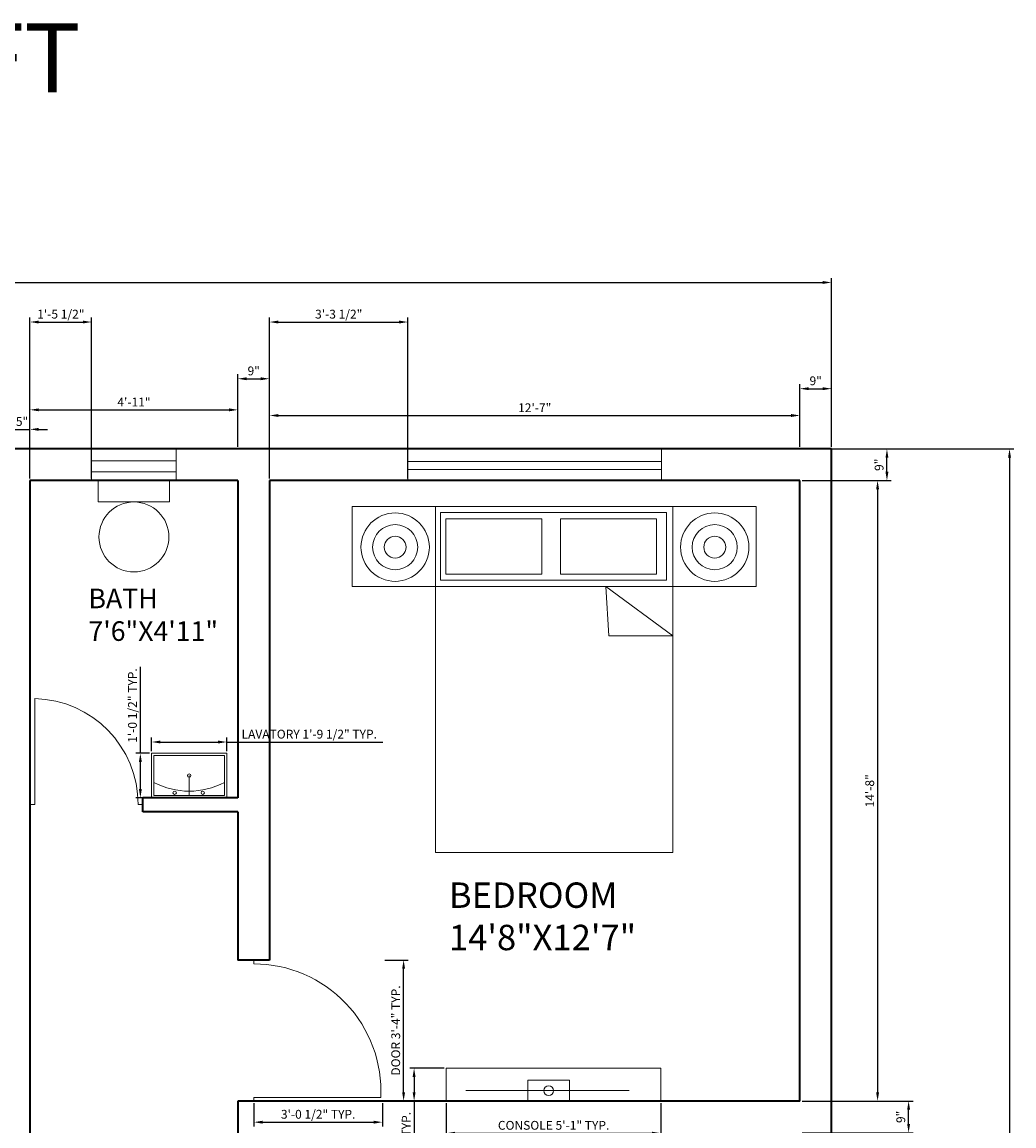
# Model space of a CAD drawing. Units: inches. Extents: x 808 to 1433, y 803 to 1556.
# Tile 4 of 4: x 1151 to 1433, y 1243 to 1556. Entities that reach past the tile are written whole.
import ezdxf

# ---------------------------------------------------------------- set-up
doc = ezdxf.new("R2010")
doc.units = ezdxf.units.IN
for name, color, linetype, lineweight in [('A-ANNO-DIMS', 7, 'Continuous', 13), ('A-AREA-IDEN', 7, 'Continuous', 18), ('A-WALL', 7, 'Continuous', 35)]:
    doc.layers.add(name, color=color, linetype=linetype, lineweight=lineweight)
for name, color, linetype, lineweight, true_color in [('A-ANNO-TITL', 244, 'Continuous', 25, 0x991b1e), ('A-DOOR', 251, 'Continuous', 18, 0x636466), ('A-FLOR-FIXT', 251, 'Continuous', 18, 0x636466), ('A-FURN', 251, 'Continuous', 13, 0x636466), ('A-GLAZ', 251, 'Continuous', 18, 0x636466)]:
    doc.layers.add(name, color=color, linetype=linetype, lineweight=lineweight, true_color=true_color)
doc.styles.get("Standard").update_dxf_attribs({"font": 'arial.ttf'})
doc.dimstyles.new('ISO-25', dxfattribs={"dimtxt": 2.5, "dimasz": 2.5, "dimexe": 1.25, "dimexo": 0.625, "dimtad": 1, "dimdec": 0, "dimlunit": 3, "dimtxsty": 'Standard', "dimcen": 2.5, "dimadec": 0, "dimazin": 0, "dimtfac": 1, "dimtdec": 0, "dimtmove": 0, "dimatfit": 3, "dimfxl": 1, "dimarcsym": 0})

# ---------------------------------------------------------------- blocks, each defined once
blk = doc.blocks.new('*D1')
at = {"layer": 'A-ANNO-DIMS', "color": 0, "lineweight": -2, "transparency": 16777216}
for p, q in [((854.88, 1435.69), (854.88, 1483.54)), ((857.38, 1482.29), (1378.38, 1482.29)), ((1380.88, 1435.69), (1380.88, 1483.54))]:
    blk.add_line(p, q, dxfattribs=at)
at = {"layer": 'A-ANNO-DIMS', "color": 0, "transparency": 16777216}
for points in [[(857.38, 1482.7), (857.38, 1481.87), (854.88, 1482.29)], [(1378.38, 1482.7), (1378.38, 1481.87), (1380.88, 1482.29)]]:
    blk.add_solid(points, dxfattribs=at)
at = {"layer": 'Defpoints', "color": 0, "transparency": 16777216}
for p in [(1380.88, 1482.29), (854.88, 1435.07), (1380.88, 1435.07)]:
    blk.add_point(p, dxfattribs=at)
at = {"layer": 'A-ANNO-DIMS', "color": 0, "transparency": 16777216, "insert": (1117.88, 1484.19), "char_height": 2.5, "attachment_point": 5}
blk.add_mtext('43\'-10"', dxfattribs=at)
blk = doc.blocks.new('*D2')
at = {"layer": 'A-ANNO-DIMS', "color": 0, "lineweight": -2, "transparency": 16777216}
for p, q in [((1381.5, 1435.07), (1432.64, 1435.07)), ((1431.39, 1432.57), (1431.39, 843.57)), ((1381.5, 841.07), (1432.64, 841.07))]:
    blk.add_line(p, q, dxfattribs=at)
at = {"layer": 'A-ANNO-DIMS', "color": 0, "transparency": 16777216}
for points in [[(1430.97, 1432.57), (1431.8, 1432.57), (1431.39, 1435.07)], [(1430.97, 843.57), (1431.8, 843.57), (1431.39, 841.07)]]:
    blk.add_solid(points, dxfattribs=at)
at = {"layer": 'Defpoints', "color": 0, "transparency": 16777216}
for p in [(1380.88, 1435.07), (1380.88, 841.07), (1431.39, 841.07)]:
    blk.add_point(p, dxfattribs=at)
at = {"layer": 'A-ANNO-DIMS', "color": 0, "transparency": 16777216, "insert": (1429.48, 1138.07), "char_height": 2.5, "attachment_point": 5, "rotation": 90}
blk.add_mtext('49\'-6"', dxfattribs=at)
blk = doc.blocks.new('*D7')
at = {"layer": 'A-ANNO-DIMS', "color": 0, "lineweight": -2, "transparency": 16777216}
for p, q in [((1146.38, 1440.62), (1143.88, 1440.62)), ((1148.88, 1435.69), (1148.88, 1441.87)), ((1148.88, 1440.62), (1153.38, 1440.62)), ((1153.38, 1435.69), (1153.38, 1441.87)), ((1155.88, 1440.62), (1158.38, 1440.62))]:
    blk.add_line(p, q, dxfattribs=at)
at = {"layer": 'A-ANNO-DIMS', "color": 0, "transparency": 16777216}
for points in [[(1146.38, 1441.04), (1146.38, 1440.2), (1148.88, 1440.62)], [(1155.88, 1441.04), (1155.88, 1440.2), (1153.38, 1440.62)]]:
    blk.add_solid(points, dxfattribs=at)
at = {"layer": 'Defpoints', "color": 0, "transparency": 16777216}
for p in [(1153.38, 1440.62), (1148.88, 1435.07), (1153.38, 1435.07)]:
    blk.add_point(p, dxfattribs=at)
at = {"layer": 'A-ANNO-DIMS', "color": 0, "transparency": 16777216, "insert": (1151.13, 1442.52), "char_height": 2.5, "attachment_point": 5}
blk.add_mtext('5"', dxfattribs=at)
blk = doc.blocks.new('*D8')
at = {"layer": 'A-ANNO-DIMS', "color": 0, "lineweight": -2, "transparency": 16777216}
for p, q in [((1153.38, 1435.69), (1153.38, 1447.4)), ((1212.38, 1435.69), (1212.38, 1447.4)), ((1155.88, 1446.15), (1209.88, 1446.15))]:
    blk.add_line(p, q, dxfattribs=at)
at = {"layer": 'A-ANNO-DIMS', "color": 0, "transparency": 16777216}
for points in [[(1155.88, 1446.57), (1155.88, 1445.74), (1153.38, 1446.15)], [(1209.88, 1446.57), (1209.88, 1445.74), (1212.38, 1446.15)]]:
    blk.add_solid(points, dxfattribs=at)
at = {"layer": 'Defpoints', "color": 0, "transparency": 16777216}
for p in [(1212.38, 1446.15), (1153.38, 1435.07), (1212.38, 1435.07)]:
    blk.add_point(p, dxfattribs=at)
at = {"layer": 'A-ANNO-DIMS', "color": 0, "transparency": 16777216, "insert": (1182.88, 1448.03), "char_height": 2.5, "attachment_point": 5}
blk.add_mtext('4\'-11"', dxfattribs=at)
blk = doc.blocks.new('*D9')
at = {"layer": 'A-ANNO-DIMS', "color": 0, "lineweight": -2, "transparency": 16777216}
for p, q in [((1212.38, 1435.69), (1212.38, 1456.23)), ((1221.38, 1435.69), (1221.38, 1456.23)), ((1214.88, 1454.98), (1218.88, 1454.98))]:
    blk.add_line(p, q, dxfattribs=at)
at = {"layer": 'A-ANNO-DIMS', "color": 0, "transparency": 16777216}
for points in [[(1214.88, 1455.39), (1214.88, 1454.56), (1212.38, 1454.98)], [(1218.88, 1455.39), (1218.88, 1454.56), (1221.38, 1454.98)]]:
    blk.add_solid(points, dxfattribs=at)
at = {"layer": 'Defpoints', "color": 0, "transparency": 16777216}
for p in [(1221.38, 1454.98), (1212.38, 1435.07), (1221.38, 1435.07)]:
    blk.add_point(p, dxfattribs=at)
at = {"layer": 'A-ANNO-DIMS', "color": 0, "transparency": 16777216, "insert": (1216.88, 1456.88), "char_height": 2.5, "attachment_point": 5}
blk.add_mtext('9"', dxfattribs=at)
blk = doc.blocks.new('*D10')
at = {"layer": 'A-ANNO-DIMS', "color": 0, "lineweight": -2, "transparency": 16777216}
for p, q in [((1371.88, 1435.69), (1371.88, 1453.41)), ((1380.88, 1435.69), (1380.88, 1453.41)), ((1374.38, 1452.16), (1378.38, 1452.16))]:
    blk.add_line(p, q, dxfattribs=at)
at = {"layer": 'A-ANNO-DIMS', "color": 0, "transparency": 16777216}
for points in [[(1374.38, 1452.57), (1374.38, 1451.74), (1371.88, 1452.16)], [(1378.38, 1452.57), (1378.38, 1451.74), (1380.88, 1452.16)]]:
    blk.add_solid(points, dxfattribs=at)
at = {"layer": 'Defpoints', "color": 0, "transparency": 16777216}
for p in [(1380.88, 1452.16), (1371.88, 1435.07), (1380.88, 1435.07)]:
    blk.add_point(p, dxfattribs=at)
at = {"layer": 'A-ANNO-DIMS', "color": 0, "transparency": 16777216, "insert": (1376.38, 1454.06), "char_height": 2.5, "attachment_point": 5}
blk.add_mtext('9"', dxfattribs=at)
blk = doc.blocks.new('*D11')
at = {"layer": 'A-ANNO-DIMS', "color": 0, "lineweight": -2, "transparency": 16777216}
for p, q in [((1221.38, 1435.69), (1221.38, 1445.8)), ((1223.88, 1444.55), (1369.38, 1444.55)), ((1371.88, 1435.69), (1371.88, 1445.8))]:
    blk.add_line(p, q, dxfattribs=at)
at = {"layer": 'A-ANNO-DIMS', "color": 0, "transparency": 16777216}
for points in [[(1223.88, 1444.97), (1223.88, 1444.13), (1221.38, 1444.55)], [(1369.38, 1444.97), (1369.38, 1444.13), (1371.88, 1444.55)]]:
    blk.add_solid(points, dxfattribs=at)
at = {"layer": 'Defpoints', "color": 0, "transparency": 16777216}
for p in [(1371.88, 1444.55), (1221.38, 1435.07), (1371.88, 1435.07)]:
    blk.add_point(p, dxfattribs=at)
at = {"layer": 'A-ANNO-DIMS', "color": 0, "transparency": 16777216, "insert": (1296.63, 1446.43), "char_height": 2.5, "attachment_point": 5}
blk.add_mtext('12\'-7"', dxfattribs=at)
blk = doc.blocks.new('*D20')
at = {"layer": 'A-ANNO-DIMS', "color": 0, "lineweight": -2, "transparency": 16777216}
for p, q in [((1372.5, 1435.07), (1397.84, 1435.07)), ((1396.59, 1428.57), (1396.59, 1432.57)), ((1372.5, 1426.07), (1397.84, 1426.07))]:
    blk.add_line(p, q, dxfattribs=at)
at = {"layer": 'A-ANNO-DIMS', "color": 0, "transparency": 16777216}
for points in [[(1396.18, 1432.57), (1397.01, 1432.57), (1396.59, 1435.07)], [(1396.18, 1428.57), (1397.01, 1428.57), (1396.59, 1426.07)]]:
    blk.add_solid(points, dxfattribs=at)
at = {"layer": 'Defpoints', "color": 0, "transparency": 16777216}
for p in [(1371.88, 1435.07), (1396.59, 1435.07), (1371.88, 1426.07)]:
    blk.add_point(p, dxfattribs=at)
at = {"layer": 'A-ANNO-DIMS', "color": 0, "transparency": 16777216, "insert": (1394.69, 1430.57), "char_height": 2.5, "attachment_point": 5, "rotation": 90}
blk.add_mtext('9"', dxfattribs=at)
blk = doc.blocks.new('*D21')
at = {"layer": 'A-ANNO-DIMS', "color": 0, "lineweight": -2, "transparency": 16777216}
for p, q in [((1372.5, 1250.07), (1404, 1250.07)), ((1402.75, 1243.57), (1402.75, 1247.57)), ((1372.5, 1241.07), (1404, 1241.07))]:
    blk.add_line(p, q, dxfattribs=at)
at = {"layer": 'A-ANNO-DIMS', "color": 0, "transparency": 16777216}
for points in [[(1402.33, 1247.57), (1403.16, 1247.57), (1402.75, 1250.07)], [(1402.33, 1243.57), (1403.16, 1243.57), (1402.75, 1241.07)]]:
    blk.add_solid(points, dxfattribs=at)
at = {"layer": 'Defpoints', "color": 0, "transparency": 16777216}
for p in [(1371.88, 1250.07), (1402.75, 1250.07), (1371.88, 1241.07)]:
    blk.add_point(p, dxfattribs=at)
at = {"layer": 'A-ANNO-DIMS', "color": 0, "transparency": 16777216, "insert": (1400.85, 1245.57), "char_height": 2.5, "attachment_point": 5, "rotation": 90}
blk.add_mtext('9"', dxfattribs=at)
blk = doc.blocks.new('*D26')
at = {"layer": 'A-ANNO-DIMS', "color": 0, "lineweight": -2, "transparency": 16777216}
for p, q in [((1381.5, 1426.07), (1395.19, 1426.07)), ((1393.94, 1423.57), (1393.94, 1252.57)), ((1381.5, 1250.07), (1395.19, 1250.07))]:
    blk.add_line(p, q, dxfattribs=at)
at = {"layer": 'A-ANNO-DIMS', "color": 0, "transparency": 16777216}
for points in [[(1393.52, 1423.57), (1394.36, 1423.57), (1393.94, 1426.07)], [(1393.52, 1252.57), (1394.36, 1252.57), (1393.94, 1250.07)]]:
    blk.add_solid(points, dxfattribs=at)
at = {"layer": 'Defpoints', "color": 0, "transparency": 16777216}
for p in [(1380.88, 1426.07), (1380.88, 1250.07), (1393.94, 1250.07)]:
    blk.add_point(p, dxfattribs=at)
at = {"layer": 'A-ANNO-DIMS', "color": 0, "transparency": 16777216, "insert": (1392.04, 1338.07), "char_height": 2.5, "attachment_point": 5, "rotation": 90}
blk.add_mtext('14\'-8"', dxfattribs=at)
blk = doc.blocks.new('BED-DOUBLE-NIGHTSTANDS')
for p, q in [((23.66, 75.46), (90.98, 75.46)), ((72.01, 75.46), (90.98, 61.39)), ((72.82, 61.39), (72.01, 75.46)), ((90.98, 61.39), (72.82, 61.39))]:
    blk.add_line(p, q)
for points in [[(23.66, 98.16), (0, 98.16), (0, 75.46), (23.66, 75.46)], [(23.66, 0), (90.98, 0), (90.98, 98.16), (23.66, 98.16)], [(114.63, 98.16), (90.98, 98.16), (90.98, 75.46), (114.63, 75.46)], [(25.04, 77.24), (89.23, 77.24), (89.23, 96.41), (25.04, 96.41)], [(26.57, 78.89), (53.84, 78.89), (53.84, 94.57), (26.57, 94.57)], [(59.07, 78.89), (86.35, 78.89), (86.35, 94.57), (59.07, 94.57)]]:
    blk.add_lwpolyline(points, close=True)
for centre, radius in [((12.19, 86.58), 9.7), ((102.89, 86.58), 9.7), ((12.19, 86.58), 6.41), ((102.89, 86.58), 6.41), ((12.19, 86.58), 3.11), ((102.89, 86.58), 3.11)]:
    blk.add_circle(centre, radius)
blk = doc.blocks.new('MEDIA-CONSOLE')
for q in [(6.39, 51.9), (6.39, 5.5)]:
    blk.add_line((6.39, 23.14), q)
for points in [[(9.33, 60.92), (0, 60.92), (0, 0), (9.33, 0)], [(9.33, 35.01), (3.45, 35.01), (3.45, 23.14), (9.33, 23.14)]]:
    blk.add_lwpolyline(points, close=True)
blk.add_circle((6.39, 29.07), 1.39)
blk = doc.blocks.new('WC')
blk.add_lwpolyline([(0, 19.84), (20.21, 19.84), (20.21, 25.9), (0, 25.9)], close=True)
for start, end in [(90, 270), (270, 90)]:
    blk.add_arc((10.11, 9.92), 9.92, start, end)
blk = doc.blocks.new('LAVATORY-COMPACT')
blk.add_line((10.66, 0.67), (10.66, 6.33))
for points in [[(21.33, 0), (0, 0), (0, 12.65), (21.33, 12.65)], [(20.66, 0.67), (0.67, 0.67), (0.67, 11.98), (20.66, 11.98)]]:
    blk.add_lwpolyline(points, close=True)
for centre in [(10.66, 6.33), (6.53, 1.45), (14.51, 1.45)]:
    blk.add_circle(centre, 0.492)
blk.add_arc((10.66, 23.6), 21.69, 242.5485, 297.4515)
blk = doc.blocks.new('WIN-72')
for points in [[(0, 0), (72, 0), (72, 9), (0, 9)], [(0, 5.39), (72, 5.39), (72, 3.12), (0, 3.12)]]:
    blk.add_lwpolyline(points, close=True)
blk = doc.blocks.new('WIN-24')
for p, q in [((0, 5.64), (24, 5.64)), ((0, 2.5), (24, 2.5))]:
    blk.add_line(p, q)
blk.add_lwpolyline([(0, 0), (24, 0), (24, 9), (0, 9)], close=True)
blk = doc.blocks.new('DOOR-32')
for p, q in [((1.38, 0), (1.38, 30)), ((1.38, 0), (0, 0)), ((32, 0), (30.69, 0))]:
    blk.add_line(p, q)
blk.add_arc((0.68, 0), 30.01, 0, 88.664)
blk = doc.blocks.new('DOOR-40')
for p, q in [((0, 40), (0, 38.9)), ((0, 1), (36, 1)), ((0, 1), (0, 0))]:
    blk.add_line(p, q)
blk.add_arc((0, 2.85), 36.05, 357.0527, 90)
blk = doc.blocks.new('*D47')
at = {"layer": 'A-ANNO-DIMS', "color": 0, "lineweight": -2, "transparency": 16777216}
for p, q in [((1254.05, 1290.07), (1260.67, 1290.07)), ((1259.42, 1252.57), (1259.42, 1287.57)), ((1254.05, 1250.07), (1260.67, 1250.07))]:
    blk.add_line(p, q, dxfattribs=at)
at = {"layer": 'A-ANNO-DIMS', "color": 0, "transparency": 16777216}
for points in [[(1259, 1287.57), (1259.84, 1287.57), (1259.42, 1290.07)], [(1259, 1252.57), (1259.84, 1252.57), (1259.42, 1250.07)]]:
    blk.add_solid(points, dxfattribs=at)
at = {"layer": 'Defpoints', "color": 0, "transparency": 16777216}
for p in [(1253.42, 1290.07), (1259.42, 1290.07), (1253.42, 1250.07)]:
    blk.add_point(p, dxfattribs=at)
at = {"layer": 'A-ANNO-DIMS', "color": 0, "transparency": 16777216, "insert": (1257.5, 1270.07), "char_height": 2.5, "attachment_point": 5, "rotation": 90}
blk.add_mtext('DOOR 3\'-4" TYP.', dxfattribs=at)
blk = doc.blocks.new('*D48')
at = {"layer": 'A-ANNO-DIMS', "color": 0, "lineweight": -2, "transparency": 16777216}
for p, q in [((1216.91, 1249.44), (1216.91, 1242.82)), ((1253.42, 1249.44), (1253.42, 1242.82)), ((1219.41, 1244.07), (1250.92, 1244.07))]:
    blk.add_line(p, q, dxfattribs=at)
at = {"layer": 'A-ANNO-DIMS', "color": 0, "transparency": 16777216}
for points in [[(1219.41, 1244.48), (1219.41, 1243.65), (1216.91, 1244.07)], [(1250.92, 1244.48), (1250.92, 1243.65), (1253.42, 1244.07)]]:
    blk.add_solid(points, dxfattribs=at)
at = {"layer": 'Defpoints', "color": 0, "transparency": 16777216}
for p in [(1216.91, 1250.07), (1253.42, 1250.07), (1253.42, 1244.07)]:
    blk.add_point(p, dxfattribs=at)
at = {"layer": 'A-ANNO-DIMS', "color": 0, "transparency": 16777216, "insert": (1235.17, 1245.98), "char_height": 2.5, "attachment_point": 5}
blk.add_mtext('3\'-0 1/2" TYP.', dxfattribs=at)
blk = doc.blocks.new('*D53')
at = {"layer": 'A-ANNO-DIMS', "color": 0, "lineweight": -2, "transparency": 16777216}
for p, q in [((1187.9, 1349.34), (1187.9, 1353.17)), ((1209.23, 1349.34), (1209.23, 1353.17)), ((1190.4, 1351.92), (1206.73, 1351.92)), ((1209.23, 1351.92), (1253.53, 1351.92))]:
    blk.add_line(p, q, dxfattribs=at)
at = {"layer": 'A-ANNO-DIMS', "color": 0, "transparency": 16777216}
for points in [[(1190.4, 1352.33), (1190.4, 1351.5), (1187.9, 1351.92)], [(1206.73, 1352.33), (1206.73, 1351.5), (1209.23, 1351.92)]]:
    blk.add_solid(points, dxfattribs=at)
at = {"layer": 'Defpoints', "color": 0, "transparency": 16777216}
for p in [(1209.23, 1351.92), (1187.9, 1348.72), (1209.23, 1348.72)]:
    blk.add_point(p, dxfattribs=at)
at = {"layer": 'A-ANNO-DIMS', "color": 0, "transparency": 16777216, "insert": (1232.63, 1353.83), "char_height": 2.5, "attachment_point": 5}
blk.add_mtext('LAVATORY 1\'-9 1/2" TYP.', dxfattribs=at)
blk = doc.blocks.new('*D54')
at = {"layer": 'A-ANNO-DIMS', "color": 0, "lineweight": -2, "transparency": 16777216}
for p, q in [((1184.7, 1348.72), (1184.7, 1373.29)), ((1187.27, 1348.72), (1183.45, 1348.72)), ((1184.7, 1338.57), (1184.7, 1346.22)), ((1187.27, 1336.07), (1183.45, 1336.07))]:
    blk.add_line(p, q, dxfattribs=at)
at = {"layer": 'A-ANNO-DIMS', "color": 0, "transparency": 16777216}
for points in [[(1184.28, 1346.22), (1185.12, 1346.22), (1184.7, 1348.72)], [(1184.28, 1338.57), (1185.12, 1338.57), (1184.7, 1336.07)]]:
    blk.add_solid(points, dxfattribs=at)
at = {"layer": 'Defpoints', "color": 0, "transparency": 16777216}
for p in [(1184.7, 1348.72), (1187.9, 1348.72), (1187.9, 1336.07)]:
    blk.add_point(p, dxfattribs=at)
at = {"layer": 'A-ANNO-DIMS', "color": 0, "transparency": 16777216, "insert": (1182.78, 1362.26), "char_height": 2.5, "attachment_point": 5, "rotation": 90}
blk.add_mtext('1\'-0 1/2" TYP.', dxfattribs=at)
blk = doc.blocks.new('*D57')
at = {"layer": 'A-ANNO-DIMS', "color": 0, "lineweight": -2, "transparency": 16777216}
for p, q in [((1271.53, 1249.44), (1271.53, 1239.68)), ((1332.45, 1249.44), (1332.45, 1239.68)), ((1274.03, 1240.93), (1329.95, 1240.93))]:
    blk.add_line(p, q, dxfattribs=at)
at = {"layer": 'A-ANNO-DIMS', "color": 0, "transparency": 16777216}
for points in [[(1274.03, 1241.35), (1274.03, 1240.51), (1271.53, 1240.93)], [(1329.95, 1241.35), (1329.95, 1240.51), (1332.45, 1240.93)]]:
    blk.add_solid(points, dxfattribs=at)
at = {"layer": 'Defpoints', "color": 0, "transparency": 16777216}
for p in [(1271.53, 1250.07), (1332.45, 1250.07), (1332.45, 1240.93)]:
    blk.add_point(p, dxfattribs=at)
at = {"layer": 'A-ANNO-DIMS', "color": 0, "transparency": 16777216, "insert": (1301.99, 1242.85), "char_height": 2.5, "attachment_point": 5}
blk.add_mtext('CONSOLE 5\'-1" TYP.', dxfattribs=at)
blk = doc.blocks.new('*D58')
at = {"layer": 'A-ANNO-DIMS', "color": 0, "lineweight": -2, "transparency": 16777216}
for p, q in [((1270.91, 1259.4), (1261.14, 1259.4)), ((1262.39, 1256.9), (1262.39, 1252.57)), ((1270.91, 1250.07), (1261.14, 1250.07)), ((1262.39, 1250.07), (1262.39, 1225.25))]:
    blk.add_line(p, q, dxfattribs=at)
at = {"layer": 'A-ANNO-DIMS', "color": 0, "transparency": 16777216}
for points in [[(1261.98, 1256.9), (1262.81, 1256.9), (1262.39, 1259.4)], [(1261.98, 1252.57), (1262.81, 1252.57), (1262.39, 1250.07)]]:
    blk.add_solid(points, dxfattribs=at)
at = {"layer": 'Defpoints', "color": 0, "transparency": 16777216}
for p in [(1271.53, 1259.4), (1262.39, 1250.07), (1271.53, 1250.07)]:
    blk.add_point(p, dxfattribs=at)
at = {"layer": 'A-ANNO-DIMS', "color": 0, "transparency": 16777216, "insert": (1260.48, 1236.41), "char_height": 2.5, "attachment_point": 5, "rotation": 90}
blk.add_mtext('0\'-9 1/2" TYP.', dxfattribs=at)
blk = doc.blocks.new('*D69')
at = {"layer": 'A-ANNO-DIMS', "color": 0, "lineweight": -2, "transparency": 16777216}
for p, q in [((1221.38, 1426.69), (1221.38, 1472.32)), ((1260.63, 1426.69), (1260.63, 1472.32)), ((1223.88, 1471.07), (1258.13, 1471.07))]:
    blk.add_line(p, q, dxfattribs=at)
at = {"layer": 'A-ANNO-DIMS', "color": 0, "transparency": 16777216}
for points in [[(1223.88, 1471.48), (1223.88, 1470.65), (1221.38, 1471.07)], [(1258.13, 1471.48), (1258.13, 1470.65), (1260.63, 1471.07)]]:
    blk.add_solid(points, dxfattribs=at)
at = {"layer": 'Defpoints', "color": 0, "transparency": 16777216}
for p in [(1260.63, 1471.07), (1221.38, 1426.07), (1260.63, 1426.07)]:
    blk.add_point(p, dxfattribs=at)
at = {"layer": 'A-ANNO-DIMS', "color": 0, "transparency": 16777216, "insert": (1241, 1472.98), "char_height": 2.5, "attachment_point": 5}
blk.add_mtext('3\'-3 1/2"', dxfattribs=at)
blk = doc.blocks.new('*D73')
at = {"layer": 'A-ANNO-DIMS', "color": 0, "lineweight": -2, "transparency": 16777216}
for p, q in [((1153.38, 1426.69), (1153.38, 1472.32)), ((1170.88, 1426.69), (1170.88, 1472.32)), ((1155.88, 1471.07), (1168.38, 1471.07))]:
    blk.add_line(p, q, dxfattribs=at)
at = {"layer": 'A-ANNO-DIMS', "color": 0, "transparency": 16777216}
for points in [[(1155.88, 1471.48), (1155.88, 1470.65), (1153.38, 1471.07)], [(1168.38, 1471.48), (1168.38, 1470.65), (1170.88, 1471.07)]]:
    blk.add_solid(points, dxfattribs=at)
at = {"layer": 'Defpoints', "color": 0, "transparency": 16777216}
for p in [(1170.88, 1471.07), (1153.38, 1426.07), (1170.88, 1426.07)]:
    blk.add_point(p, dxfattribs=at)
at = {"layer": 'A-ANNO-DIMS', "color": 0, "transparency": 16777216, "insert": (1162.13, 1472.98), "char_height": 2.5, "attachment_point": 5}
blk.add_mtext('1\'-5 1/2"', dxfattribs=at)

msp = doc.modelspace()

# ---------------------------------------------------------------- linework, layer by layer
at = {"layer": 'A-WALL'}
for p, q in [((1380.88, 1435.07), (854.88, 1435.07)), ((1380.88, 841.07), (1380.88, 1435.07)), ((1153.38, 1426.07), (1153.38, 1332.07)), ((1212.38, 1426.07), (1153.38, 1426.07)), ((1212.38, 1426.07), (1212.38, 1336.07)), ((1371.88, 1426.07), (1221.38, 1426.07)), ((1221.38, 1426.07), (1221.38, 1290.07)), ((1371.88, 1250.07), (1371.88, 1426.07)), ((1212.38, 1336.07), (1185.38, 1336.07)), ((1185.38, 1332.07), (1185.38, 1336.07)), ((1153.38, 1332.07), (1153.38, 1241.07)), ((1212.38, 1332.07), (1185.38, 1332.07)), ((1212.38, 1332.07), (1212.38, 1290.07)), ((1221.38, 1290.07), (1212.38, 1290.07)), ((1371.88, 1250.07), (1212.38, 1250.07)), ((1212.38, 1250.07), (1212.38, 1241.07))]:
    msp.add_line(p, q, dxfattribs=at)

# ---------------------------------------------------------------- block references
at = {"layer": 'A-DOOR'}
for name, p in [('DOOR-32', (1153.38, 1334.23)), ('DOOR-40', (1216.91, 1250.07))]:
    msp.add_blockref(name, p, dxfattribs=at)
at = {"layer": 'A-FLOR-FIXT'}
for name, p in [('WC', (1172.77, 1400.17)), ('LAVATORY-COMPACT', (1187.9, 1336.07))]:
    msp.add_blockref(name, p, dxfattribs=at)
at = {"layer": 'A-FURN'}
msp.add_blockref('BED-DOUBLE-NIGHTSTANDS', (1244.83, 1320.62), dxfattribs=at)
at = {"layer": 'A-FURN', "rotation": 270.0000000000009}
msp.add_blockref('MEDIA-CONSOLE', (1271.53, 1259.4), dxfattribs=at)
at = {"layer": 'A-GLAZ'}
for name, p in [('WIN-24', (1170.88, 1426.07)), ('WIN-72', (1260.63, 1426.07))]:
    msp.add_blockref(name, p, dxfattribs=at)

# ---------------------------------------------------------------- texts
at = {"layer": 'A-ANNO-TITL', "insert": (1031.76, 1555.82), "char_height": 19.557, "attachment_point": 1}
msp.add_mtext_dynamic_manual_height_columns('43FTX49FT', width=1471.4106, gutter_width=97.78, heights=[0], dxfattribs=at)
at = {"layer": 'A-AREA-IDEN', "attachment_point": 1}
for s, width, gutter_width, insert, char_height in [('BATH\\P7\'6"X4\'11"', 53.1011, 27.79, (1169.97, 1395.43), 5.557), ('BEDROOM\\P14\'8"X12\'7"', 312.5212, 36.01, (1272.28, 1312.07), 7.2014)]:
    msp.add_mtext_dynamic_manual_height_columns(s, width=width, gutter_width=gutter_width, heights=[0], dxfattribs=dict(at, insert=insert, char_height=char_height))

# ---------------------------------------------------------------- dimensions: what is measured, and where the dimension line sits
at = {"layer": 'A-ANNO-DIMS'}
for base, p1, p2, override, picture, middle in [((1380.88, 1482.29), (854.88, 1435.07), (1380.88, 1435.07), {"dimclrd": 0, "dimclre": 0, "dimclrt": 0}, '*D1', (1117.88, 1484.19)), ((1170.88, 1471.07), (1153.38, 1426.07), (1170.88, 1426.07), {"dimdec": 1, "dimlfac": 1, "dimrnd": 0, "dimzin": 1, "dimdsep": 46, "dimlunit": 4, "dimfrac": 2}, '*D73', (1162.13, 1472.98)), ((1260.629538, 1471.06624), (1221.379538, 1426.06624), (1260.629538, 1426.06624), {"dimdec": 1, "dimlfac": 1, "dimrnd": 0, "dimzin": 1, "dimdsep": 46, "dimlunit": 4, "dimfrac": 2}, '*D69', (1241.004538, 1472.98472568)), ((1221.38, 1454.98), (1212.38, 1435.07), (1221.38, 1435.07), {"dimclrd": 0, "dimclre": 0, "dimclrt": 0}, '*D9', (1216.88, 1456.88)), ((1380.88, 1452.16), (1371.88, 1435.07), (1380.88, 1435.07), {"dimclrd": 0, "dimclre": 0, "dimclrt": 0}, '*D10', (1376.38, 1454.06)), ((1212.38, 1446.15), (1153.38, 1435.07), (1212.38, 1435.07), {"dimclrd": 0, "dimclre": 0, "dimclrt": 0}, '*D8', (1182.88, 1448.03)), ((1371.87953788, 1444.54957373), (1221.37953788, 1435.06624021), (1371.87953788, 1435.06624021), {"dimclrd": 0, "dimclre": 0, "dimclrt": 0}, '*D11', (1296.62953788, 1446.4296897)), ((1153.37953788, 1440.61951025), (1148.87953788, 1435.06624021), (1153.37953788, 1435.06624021), {"dimclrd": 0, "dimclre": 0, "dimclrt": 0}, '*D7', (1151.12953788, 1442.51582676))]:
    dim = msp.add_linear_dim(base=base, p1=p1, p2=p2, dimstyle='ISO-25', override=override, dxfattribs=at)
    dim.commit()
    dim.dimension.update_dxf_attribs({"geometry": picture, "text_midpoint": middle})
for base, p1, p2, picture, middle in [((1396.59, 1435.07), (1371.88, 1426.07), (1371.88, 1435.07), '*D20', (1394.69, 1430.57)), ((1431.39, 841.07), (1380.88, 1435.07), (1380.88, 841.07), '*D2', (1429.48, 1138.07)), ((1393.94, 1250.07), (1380.88, 1426.07), (1380.88, 1250.07), '*D26', (1392.04, 1338.07)), ((1402.75, 1250.07), (1371.88, 1241.07), (1371.88, 1250.07), '*D21', (1400.85, 1245.57))]:
    dim = msp.add_linear_dim(base=base, p1=p1, p2=p2, angle=90, dimstyle='ISO-25', override={"dimclrd": 0, "dimclre": 0, "dimclrt": 0}, dxfattribs=at)
    dim.commit()
    dim.dimension.update_dxf_attribs({"geometry": picture, "text_midpoint": middle})
for base, p1, p2, angle, text, picture, middle in [((1184.6993, 1348.71618), (1187.89875, 1336.06624), (1187.89875, 1348.71618), 90, '<> TYP.', '*D54', (1182.78166, 1362.25557)), ((1259.42, 1290.07), (1253.42, 1250.07), (1253.42, 1290.07), 90, 'DOOR <> TYP.', '*D47', (1257.5, 1270.07)), ((1262.39, 1250.07), (1271.53, 1259.4), (1271.53, 1250.07), 270, '<> TYP.', '*D58', (1260.48, 1236.41)), ((1332.45, 1240.93), (1271.53, 1250.07), (1332.45, 1250.07), 0, 'CONSOLE <> TYP.', '*D57', (1301.99, 1242.85))]:
    dim = msp.add_linear_dim(base=base, p1=p1, p2=p2, angle=angle, text=text, dimstyle='ISO-25', override={"dimdec": 1, "dimlfac": 1, "dimrnd": 0, "dimzin": 1, "dimdsep": 46, "dimlunit": 4, "dimfrac": 2}, dxfattribs=at)
    dim.commit()
    dim.dimension.update_dxf_attribs({"geometry": picture, "text_midpoint": middle})
for base, p1, p2, text, picture, middle in [((1209.23, 1351.92), (1187.9, 1348.72), (1209.23, 1348.72), 'LAVATORY <> TYP.', '*D53', (1232.63, 1353.83)), ((1253.42, 1244.07), (1216.91, 1250.07), (1253.42, 1250.07), '<> TYP.', '*D48', (1235.17, 1245.98))]:
    dim = msp.add_linear_dim(base=base, p1=p1, p2=p2, text=text, dimstyle='ISO-25', override={"dimdec": 1, "dimlfac": 1, "dimrnd": 0, "dimzin": 1, "dimdsep": 46, "dimlunit": 4, "dimfrac": 2}, dxfattribs=at)
    dim.commit()
    dim.dimension.update_dxf_attribs({"geometry": picture, "text_midpoint": middle})

doc.saveas('drawing.dxf')
